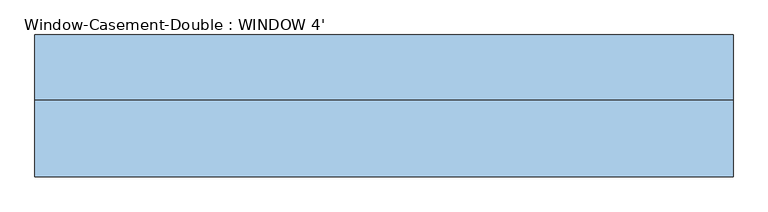
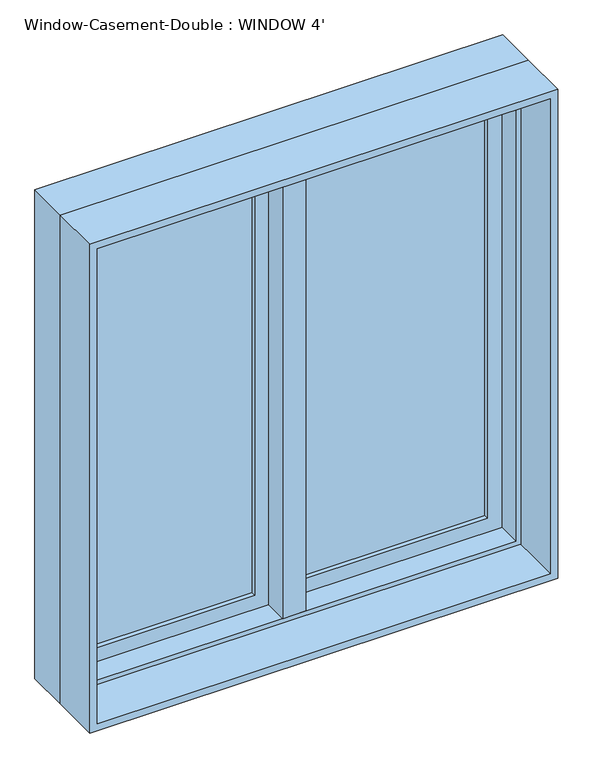
"""IFC4 building model written with IfcOpenShell, lengths in millimetres: window geometry, Window-Casement-Double : WINDOW 4'."""

from ifc_helpers import new_model, si_unit, frame, origin, place, context, project, spatial, polyline, outline, extrude, faceted_brep, source, transform, mapped, element, save


def window_casement_double_window_4_576b2d2c(model_context):
    return source(origin(), model_context, "Body", "SolidModel", [
        faceted_brep([(9.525, 133.35, 2247.9), (-9.525, 133.35, 2247.9), (-9.525, 82.55, 2247.9), (9.525, 82.55, 2247.9), (9.525, 133.35, 927.1), (9.525, 82.55, 927.1), (-9.525, 82.55, 927.1), (-9.525, 133.35, 927.1), (-9.525, 82.55, 946.15), (-9.525, 82.55, 2228.85), (-30.1625, 82.55, 946.15), (-30.1625, 82.55, 2228.85), (-30.1625, 19.05, 946.15), (-30.1625, 19.05, 2228.85), (30.1625, 19.05, 946.15), (30.1625, 19.05, 2228.85), (30.1625, 82.55, 946.15), (30.1625, 82.55, 2228.85), (9.525, 82.55, 946.15), (9.525, 82.55, 2228.85)], [[[0, 1, 2, 3]], [[4, 5, 6, 7]], [[1, 0, 4, 7]], [[2, 1, 7, 6, 8, 9]], [[9, 8, 10, 11]], [[11, 10, 12, 13]], [[13, 12, 14, 15]], [[15, 14, 16, 17]], [[17, 16, 18, 19]], [[0, 3, 19, 18, 5, 4]], [[18, 8, 6, 5]], [[9, 19, 3, 2]], [[8, 18, 16, 14, 12, 10]], [[19, 9, 11, 13, 15, 17]]]),
        extrude(outline(polyline([(-66.675, 114.3), (-66.675, 107.95), (-539.75, 107.95), (-539.75, 114.3), (-66.675, 114.3)])), frame((0.0, 0.0, 984.25), z_axis=(0.0, 0.0, 1.0), x_axis=(1.0, 0.0, 0.0)), (0.0, 0.0, 1.0), 1206.5),
        extrude(outline(polyline([(-539.75, 95.25), (-539.75, 101.6), (-66.675, 101.6), (-66.675, 95.25), (-539.75, 95.25)])), frame((0.0, 0.0, 984.25), z_axis=(0.0, 0.0, 1.0), x_axis=(1.0, 0.0, 0.0)), (0.0, 0.0, 1.0), 1206.5),
        extrude(outline(polyline([(539.75, 114.3), (539.75, 107.95), (66.675, 107.95), (66.675, 114.3), (539.75, 114.3)])), frame((0.0, 0.0, 984.25), z_axis=(0.0, 0.0, 1.0), x_axis=(1.0, 0.0, 0.0)), (0.0, 0.0, 1.0), 1206.5),
        extrude(outline(polyline([(66.675, 95.25), (66.675, 101.6), (539.75, 101.6), (539.75, 95.25), (66.675, 95.25)])), frame((0.0, 0.0, 984.25), z_axis=(0.0, 0.0, 1.0), x_axis=(1.0, 0.0, 0.0)), (0.0, 0.0, 1.0), 1206.5),
        extrude(outline(polyline([(2247.9, -596.9), (927.1, -596.9), (927.1, -9.525), (2247.9, -9.525), (2247.9, -596.9)]), holes=[polyline([(2190.75, -66.675), (984.25, -66.675), (984.25, -539.75), (2190.75, -539.75), (2190.75, -66.675)])]), frame((0.0, 82.55, 0.0), z_axis=(0.0, 1.0, 0.0), x_axis=(0.0, 0.0, 1.0)), (0.0, 0.0, 1.0), 44.45),
        extrude(outline(polyline([(927.1, 596.9), (2247.9, 596.9), (2247.9, 9.525), (927.1, 9.525), (927.1, 596.9)]), holes=[polyline([(984.25, 66.675), (2190.75, 66.675), (2190.75, 539.75), (984.25, 539.75), (984.25, 66.675)])]), frame((0.0, 82.55, 0.0), z_axis=(0.0, 1.0, 0.0), x_axis=(0.0, 0.0, 1.0)), (0.0, 0.0, 1.0), 44.45),
        extrude(outline(polyline([(2260.6, -609.6), (914.4, -609.6), (914.4, 609.6), (2260.6, 609.6), (2260.6, -609.6)]), holes=[polyline([(2241.55, 590.55), (933.45, 590.55), (933.45, -590.55), (2241.55, -590.55), (2241.55, 590.55)])]), frame((0.0, -114.3, 0.0), z_axis=(0.0, 1.0, 0.0), x_axis=(0.0, 0.0, 1.0)), (0.0, 0.0, 1.0), 133.35),
        faceted_brep([(577.85, 82.55, 2228.85), (577.85, 19.05, 2228.85), (-577.85, 19.05, 2228.85), (-577.85, 82.55, 2228.85), (596.9, 133.35, 2247.9), (596.9, 82.55, 2247.9), (-596.9, 82.55, 2247.9), (-596.9, 133.35, 2247.9), (609.6, 19.05, 2260.6), (609.6, 133.35, 2260.6), (-609.6, 133.35, 2260.6), (-609.6, 19.05, 2260.6), (-577.85, 19.05, 946.15), (-577.85, 82.55, 946.15), (-596.9, 82.55, 927.1), (-596.9, 133.35, 927.1), (-609.6, 133.35, 914.4), (-609.6, 19.05, 914.4), (577.85, 19.05, 946.15), (577.85, 82.55, 946.15), (596.9, 82.55, 927.1), (596.9, 133.35, 927.1), (609.6, 133.35, 914.4), (609.6, 19.05, 914.4)], [[[0, 1, 2, 3]], [[4, 5, 6, 7]], [[8, 9, 10, 11]], [[3, 2, 12, 13]], [[7, 6, 14, 15]], [[11, 10, 16, 17]], [[13, 12, 18, 19]], [[15, 14, 20, 21]], [[17, 16, 22, 23]], [[11, 17, 23, 8], [1, 18, 12, 2]], [[19, 18, 1, 0]], [[5, 20, 14, 6], [3, 13, 19, 0]], [[21, 20, 5, 4]], [[23, 22, 9, 8]], [[9, 22, 16, 10], [7, 15, 21, 4]]]),
    ])


if __name__ == "__main__":
    model = new_model("IFC4")
    model_context = context("Model", 3, world=origin())
    ifc_project = project(units=[si_unit("LENGTHUNIT", "METRE", prefix="MILLI")], contexts=[model_context])
    site = spatial("IfcSite", under=ifc_project)
    building = spatial("IfcBuilding", under=site)
    placement = place(None, origin())
    window_casement_double_window_4_shape = window_casement_double_window_4_576b2d2c(model_context)
    element("IfcWindow", 1, ObjectType="Window-Casement-Double : WINDOW 4'", at=placement, inside=building, context=model_context, shape_type="MappedRepresentation", body=[
        mapped(window_casement_double_window_4_shape, transform((0.0, 0.0, 0.0), x_axis=(1.0, 0.0, 0.0), y_axis=(0.0, 1.0, 0.0), z_axis=(0.0, 0.0, 1.0))),
    ])
    save(model, "model.ifc")

# Revit data of these elements
# Type "Window-Casement-Double : WINDOW 4'"
#   Type Mark = "18"
#   Fire Rating = "0.5h"
#   Assembly Code = "B2020100"
#   Analytic Construction = "Double glazing - domestic"
#   Frame Extension [instance default] = 0' - 0 1/4"
#   Window Inset [instance default] = 0' - 0"
#   Wall Thickness [instance default] = 0' - 6"
#   Interior Wall Closure [instance default] = 0' - 2 1/4"
#   Half Width = 2' - 0"
#   Visual Light Transmittance = 0.81
#   Thermal Resistance (R) = 1.8146 (h·ft²·°F)/BTU
#   Solar Heat Gain Coefficient = 0.76
#   Rough Width = 4' - 0 1/2"
#   Rough Height = 4' - 5 1/2"
#   Height = 4' - 5"
#   Heat Transfer Coefficient (U) = 0.5511 BTU/(h·ft²·°F)
#   Exterior Wall Closure [instance default] = 0' - 1 1/4"
#   Extension Jamb [instance default] = 0' - 2 1/4"
#   Default Sill Height = 3' - 0"
#   Width = 4' - 0"
#   Muntin Visibility = yes
#   Interior Trim Visibility [instance default] = yes
#   Exterior Trim Visibility [instance default] = yes
#   Extension Jamb Visibility [instance default] = yes
#   Interior Trim Material = Wood - Stained
#   Muntin Pattern = Muntin Pattern_2x2 : Muntin Pattern_2x2
#   Interior Trim = Trim-Window-Interior-Flat : Picture Frame
#   Interior Frame Material = Wood - Stained
#   Glass Panel Material = Glass
#   Exterior Trim Material = Clad - White
#   Exterior Trim = Trim-Window-Exterior-Flat : with Sill
#   Exterior Frame Material = Clad - White
#   Wall Closure = (empty or 0)
# Element 1 (IfcWindow, "Window-Casement-Double : WINDOW 4'")
#   Wall Thickness = 0' - 9"
#   Extension Jamb = 0' - 5 1/4"
#   Materials on its faces: "Wood - Stained", "Glass", "Clad - White"
# Materials
#   "Wood - Stained": class "Wood", colour RGB 224 178 126, transparency 0, Cost = 0
#   "Glass": class "Glass", colour RGB 0 128 192, transparency 0.75, Description = "Soda Lime Glass", Cost = 0
#   "Clad - White": class "Wood", colour RGB 242 242 238, transparency 0, Cost = 0
